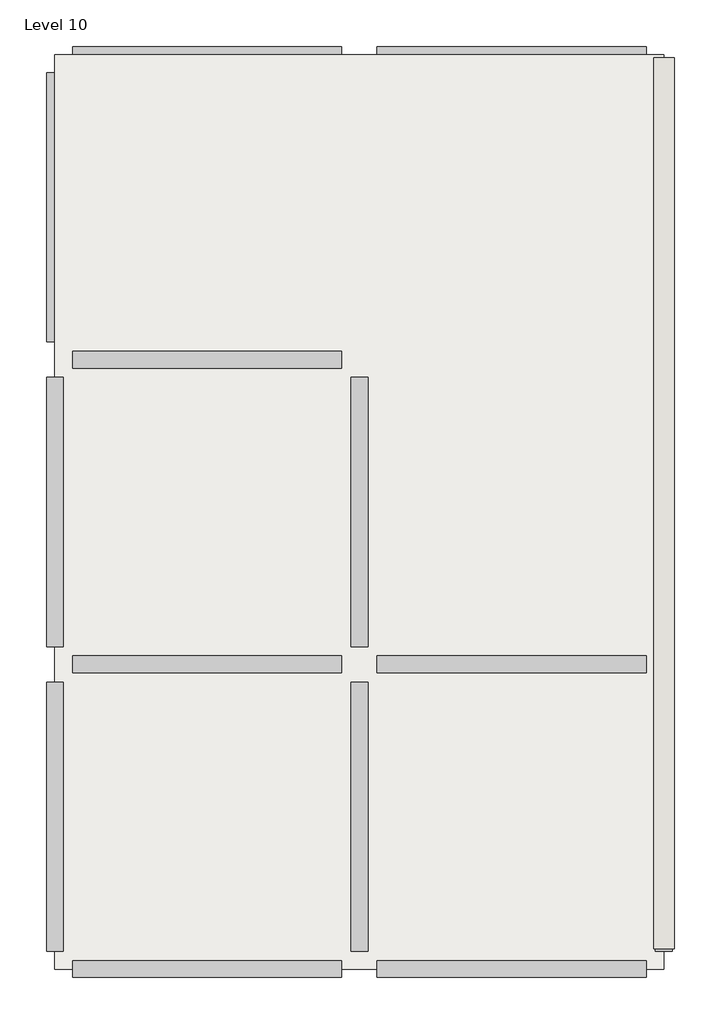
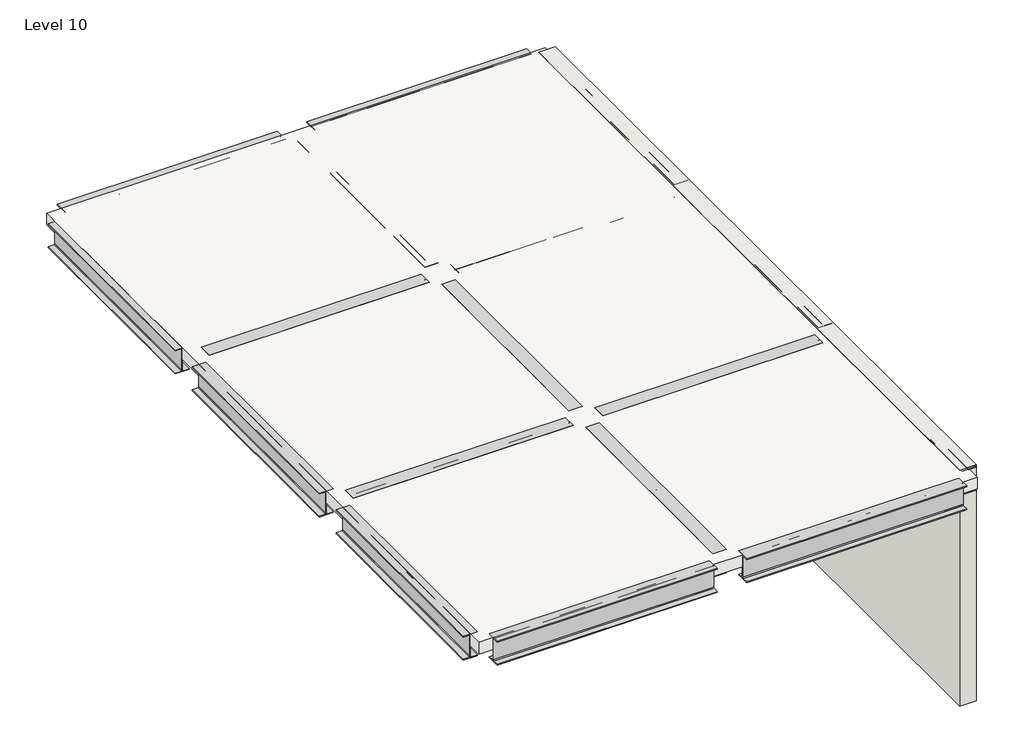
# One storey: 17 beams, 1 slab, 1 wall.
"""IFC4 building model written with IfcOpenShell, lengths in millimetres."""

from ifc_helpers import new_model, si_unit, frame, origin, place, context, project, spatial, polyline, outline, extrude, transform, mapped, element, save
from components import ub_universal_beams_ub305x165x40_60ab2ee1

model = new_model("IFC4")

# Units and contexts
model_context = context("Model", 3, world=origin())
ifc_project = project(units=[si_unit("LENGTHUNIT", "METRE", prefix="MILLI")], contexts=[model_context])

# Site, building, storey
site = spatial("IfcSite", under=ifc_project)
building = spatial("IfcBuilding", under=site)
storey = spatial("IfcBuildingStorey", under=building, Name="Level 10", Elevation=27000.0)

# Beams
placement = place(None, origin())
ub_universal_beams_ub305x165x40_shape = ub_universal_beams_ub305x165x40_60ab2ee1(model_context)
element("IfcBeam", 1, ObjectType="UB-Universal Beams : UB305x165x40", at=placement, inside=storey, context=model_context, shape_type="MappedRepresentation", body=[
    mapped(ub_universal_beams_ub305x165x40_shape, transform((18435.1404262, -6314.7314166, 26848.3), x_axis=(-1.0, 0.0, 0.0), y_axis=(0.0, -1.0, 0.0), z_axis=(0.0, 0.0, 1.0))),
])
element("IfcBeam", 2, ObjectType="UB-Universal Beams : UB305x165x40", at=placement, inside=storey, context=model_context, shape_type="MappedRepresentation", body=[
    mapped(ub_universal_beams_ub305x165x40_shape, transform((15435.1404262, -6314.7314166, 26848.3), x_axis=(-1.0, 0.0, 0.0), y_axis=(0.0, -1.0, 0.0), z_axis=(0.0, 0.0, 1.0))),
])
element("IfcBeam", 3, ObjectType="UB-Universal Beams : UB305x165x40", at=placement, inside=storey, context=model_context, shape_type="MappedRepresentation", body=[
    mapped(ub_universal_beams_ub305x165x40_shape, transform((13935.1404262, -4814.7314166, 26848.3), x_axis=(0.0, 1.0, 0.0), y_axis=(-1.0, 0.0, 0.0), z_axis=(0.0, 0.0, 1.0))),
])
element("IfcBeam", 4, ObjectType="UB-Universal Beams : UB305x165x40", at=placement, inside=storey, context=model_context, shape_type="MappedRepresentation", body=[
    mapped(ub_universal_beams_ub305x165x40_shape, transform((13935.1404262, -1814.7314166, 26848.3), x_axis=(0.0, 1.0, 0.0), y_axis=(-1.0, 0.0, 0.0), z_axis=(0.0, 0.0, 1.0))),
])
element("IfcBeam", 5, ObjectType="UB-Universal Beams : UB305x165x40", at=placement, inside=storey, context=model_context, shape_type="MappedRepresentation", body=[
    mapped(ub_universal_beams_ub305x165x40_shape, transform((13935.1404262, 1185.2685834, 26848.3), x_axis=(0.0, 1.0, 0.0), y_axis=(-1.0, 0.0, 0.0), z_axis=(0.0, 0.0, 1.0))),
])
element("IfcBeam", 6, ObjectType="UB-Universal Beams : UB305x165x40", at=placement, inside=storey, context=model_context, shape_type="MappedRepresentation", body=[
    mapped(ub_universal_beams_ub305x165x40_shape, transform((18435.1404262, -3314.7314166, 26848.3), x_axis=(-1.0, 0.0, 0.0), y_axis=(0.0, -1.0, 0.0), z_axis=(0.0, 0.0, 1.0))),
])
element("IfcBeam", 7, ObjectType="UB-Universal Beams : UB305x165x40", at=placement, inside=storey, context=model_context, shape_type="MappedRepresentation", body=[
    mapped(ub_universal_beams_ub305x165x40_shape, transform((15435.1404262, -3314.7314166, 26848.3), x_axis=(-1.0, 0.0, 0.0), y_axis=(0.0, -1.0, 0.0), z_axis=(0.0, 0.0, 1.0))),
])
element("IfcBeam", 8, ObjectType="UB-Universal Beams : UB305x165x40", at=placement, inside=storey, context=model_context, shape_type="MappedRepresentation", body=[
    mapped(ub_universal_beams_ub305x165x40_shape, transform((18435.1404262, -314.7314166, 26848.3), x_axis=(-1.0, 0.0, 0.0), y_axis=(0.0, -1.0, 0.0), z_axis=(0.0, 0.0, 1.0))),
])
element("IfcBeam", 9, ObjectType="UB-Universal Beams : UB305x165x40", at=placement, inside=storey, context=model_context, shape_type="MappedRepresentation", body=[
    mapped(ub_universal_beams_ub305x165x40_shape, transform((15435.1404262, -314.7314166, 26848.3), x_axis=(-1.0, 0.0, 0.0), y_axis=(0.0, -1.0, 0.0), z_axis=(0.0, 0.0, 1.0))),
])
element("IfcBeam", 10, ObjectType="UB-Universal Beams : UB305x165x40", at=placement, inside=storey, context=model_context, shape_type="MappedRepresentation", body=[
    mapped(ub_universal_beams_ub305x165x40_shape, transform((18435.1404262, 2685.2685834, 26848.3), x_axis=(-1.0, 0.0, 0.0), y_axis=(0.0, -1.0, 0.0), z_axis=(0.0, 0.0, 1.0))),
])
element("IfcBeam", 11, ObjectType="UB-Universal Beams : UB305x165x40", at=placement, inside=storey, context=model_context, shape_type="MappedRepresentation", body=[
    mapped(ub_universal_beams_ub305x165x40_shape, transform((15435.1404262, 2685.2685834, 26848.3), x_axis=(-1.0, 0.0, 0.0), y_axis=(0.0, -1.0, 0.0), z_axis=(0.0, 0.0, 1.0))),
])
element("IfcBeam", 12, ObjectType="UB-Universal Beams : UB305x165x40", at=placement, inside=storey, context=model_context, shape_type="MappedRepresentation", body=[
    mapped(ub_universal_beams_ub305x165x40_shape, transform((16935.1404262, -4814.7314166, 26848.3), x_axis=(0.0, 1.0, 0.0), y_axis=(-1.0, 0.0, 0.0), z_axis=(0.0, 0.0, 1.0))),
])
element("IfcBeam", 13, ObjectType="UB-Universal Beams : UB305x165x40", at=placement, inside=storey, context=model_context, shape_type="MappedRepresentation", body=[
    mapped(ub_universal_beams_ub305x165x40_shape, transform((16935.1404262, -1814.7314166, 26848.3), x_axis=(0.0, 1.0, 0.0), y_axis=(-1.0, 0.0, 0.0), z_axis=(0.0, 0.0, 1.0))),
])
element("IfcBeam", 14, ObjectType="UB-Universal Beams : UB305x165x40", at=placement, inside=storey, context=model_context, shape_type="MappedRepresentation", body=[
    mapped(ub_universal_beams_ub305x165x40_shape, transform((16935.1404262, 1185.2685834, 26848.3), x_axis=(0.0, 1.0, 0.0), y_axis=(-1.0, 0.0, 0.0), z_axis=(0.0, 0.0, 1.0))),
])
element("IfcBeam", 15, ObjectType="UB-Universal Beams : UB305x165x40", at=placement, inside=storey, context=model_context, shape_type="MappedRepresentation", body=[
    mapped(ub_universal_beams_ub305x165x40_shape, transform((19935.1404262, -1814.7314166, 26848.3), x_axis=(0.0, 1.0, 0.0), y_axis=(-1.0, 0.0, 0.0), z_axis=(0.0, 0.0, 1.0))),
])
element("IfcBeam", 16, ObjectType="UB-Universal Beams : UB305x165x40", at=placement, inside=storey, context=model_context, shape_type="MappedRepresentation", body=[
    mapped(ub_universal_beams_ub305x165x40_shape, transform((19935.1404262, 1185.2685834, 26848.3), x_axis=(0.0, 1.0, 0.0), y_axis=(-1.0, 0.0, 0.0), z_axis=(0.0, 0.0, 1.0))),
])
element("IfcBeam", 17, ObjectType="UB-Universal Beams : beam", at=placement, inside=storey, context=model_context, shape_type="MappedRepresentation", body=[
    mapped(ub_universal_beams_ub305x165x40_shape, transform((19935.1404262, -4814.7314166, 26848.3), x_axis=(0.0, 1.0, 0.0), y_axis=(-1.0, 0.0, 0.0), z_axis=(0.0, 0.0, 1.0))),
])

# Slab
element("IfcSlab", 18, ObjectType="150mm Foundation Slab", at=placement, inside=storey, context=model_context, shape_type="SweptSolid", body=[
    extrude(outline(polyline([(13935.1404262, -6314.7314166), (13935.1404262, 2685.2685834), (19935.1404262, 2685.2685834), (19935.1404262, -6314.7314166), (13935.1404262, -6314.7314166)])), frame((0.0, 0.0, 26850.0), z_axis=(0.0, 0.0, 1.0), x_axis=(1.0, 0.0, 0.0)), (0.0, 0.0, 1.0), 150.0),
])

# Wall
element("IfcWall", 19, ObjectType="Generic - 200mm", at=placement, inside=storey, context=model_context, shape_type="SweptSolid", body=[
    extrude(outline(polyline([(19835.1404262, -6114.7314166), (19835.1404262, 2655.9792615), (20035.1404262, 2655.9792615), (20035.1404262, -6114.7314166), (19835.1404262, -6114.7314166)])), frame((0.0, 0.0, 24000.0), z_axis=(0.0, 0.0, 1.0), x_axis=(1.0, 0.0, 0.0)), (0.0, 0.0, 1.0), 3000.0),
])

save(model, "model.ifc")

# Revit data of these elements
# Type "UB-Universal Beams : UB305x165x40"
#   Section Name Key = "UB305X165X40"
#   Width = 16.5 cm
#   Web Thickness = 0.6 cm
#   Web Fillet = 0.89 cm
#   Warping Constant = 164000.0 cm⁶
#   Torsional Moment of Inertia = 14.70 cm⁴
#   Section Area = 51.3 cm²
#   Plastic Modulus weak axis = 142.0 cm³
#   Plastic Modulus strong axis = 623.0 cm³
#   Nominal Weight = 40.2999 kgf/m
#   Moment of Inertia weak axis = 764.00 cm⁴
#   Moment of Inertia strong axis = 8503.00 cm⁴
#   Height = 30.34 cm
#   Flange Thickness = 1.02 cm
#   Elastic Modulus weak axis = 92.6 cm³
#   Elastic Modulus strong axis = 560.0 cm³
#   Centroid Vertical = 15.17 cm
#   Centroid Horizontal = 8.25 cm
#   Bolt Spacing = 9.0 cm
#   Length [instance default] = 1.5 m
#   Structural Material [instance default] = Metal - Steel 43-275
#   Type Comments = ""
#   Assembly Code = ""
# Type "UB-Universal Beams : beam"
#   Section Name Key = "UB305X165X40"
#   Width = 16.5 cm
#   Web Thickness = 0.6 cm
#   Web Fillet = 0.89 cm
#   Warping Constant = 164000.0 cm⁶
#   Torsional Moment of Inertia = 14.70 cm⁴
#   Section Area = 51.3 cm²
#   Plastic Modulus weak axis = 142.0 cm³
#   Plastic Modulus strong axis = 623.0 cm³
#   Nominal Weight = 40.2999 kgf/m
#   Moment of Inertia weak axis = 764.00 cm⁴
#   Moment of Inertia strong axis = 8503.00 cm⁴
#   Height = 30.34 cm
#   Flange Thickness = 1.02 cm
#   Elastic Modulus weak axis = 92.6 cm³
#   Elastic Modulus strong axis = 560.0 cm³
#   Centroid Vertical = 15.17 cm
#   Centroid Horizontal = 8.25 cm
#   Bolt Spacing = 9.0 cm
#   Length [instance default] = 1.5 m
#   Structural Material [instance default] = Metal - Steel 43-275
#   Type Comments = ""
#   Assembly Code = ""
# Type "150mm Foundation Slab"
#   Layers, outside or top first: 0.15 m "Concrete, Cast-in-Place gray" (function 1)
# Type "Generic - 200mm"
#   Layers, outside or top first: 0.2 m no material (function 1)
# Elements 1, 2, 3, 4, 5, 6, 7, 8, 9, 10, 11, 12, 13, 14, 15, 16 (IfcBeam, "UB-Universal Beams : UB305x165x40")
#   Structural Material = Metal - Steel 43-275
#   Phase Created = New Construction
#   Materials on its faces: "Metal - Steel 43-275"
# Element 17 (IfcBeam, "UB-Universal Beams : beam")
#   Structural Material = Metal - Steel 43-275
#   Phase Created = New Construction
#   Materials on its faces: "Metal - Steel 43-275"
# Element 18 (IfcSlab, "150mm Foundation Slab")
#   built-in parameter 1001955 = 3.14159 (stored number, unit not read)
#   Height Offset From Level = 0 m
#   built-in parameter 1001954 = 1
#   Phase Created = New Construction
#   Materials on its faces: "Concrete, Cast-in-Place gray"
# Element 19 (IfcWall, "Generic - 200mm")
#   Comments = ""
#   built-in parameter 1001111 = -3 m
#   Top Offset = 0 m
#   Base Offset = -3 m
#   wall height = 3 m
#   Phase Created = New Construction
#   Base Constraint = Level 10
#   Top Constraint = Level 10
#   Materials on its faces: "Default Wall"
# Materials
#   "Metal - Steel 43-275": class "Metal", colour RGB 247 247 247, transparency 0, Cost = 0
#   "Concrete, Cast-in-Place gray": class "Concrete", colour RGB 192 192 192, transparency 0, Description = "Cast-in-place concrete", Cost = 0
#   "Default Wall": colour RGB 128 128 128, transparency 0, Cost = 0
